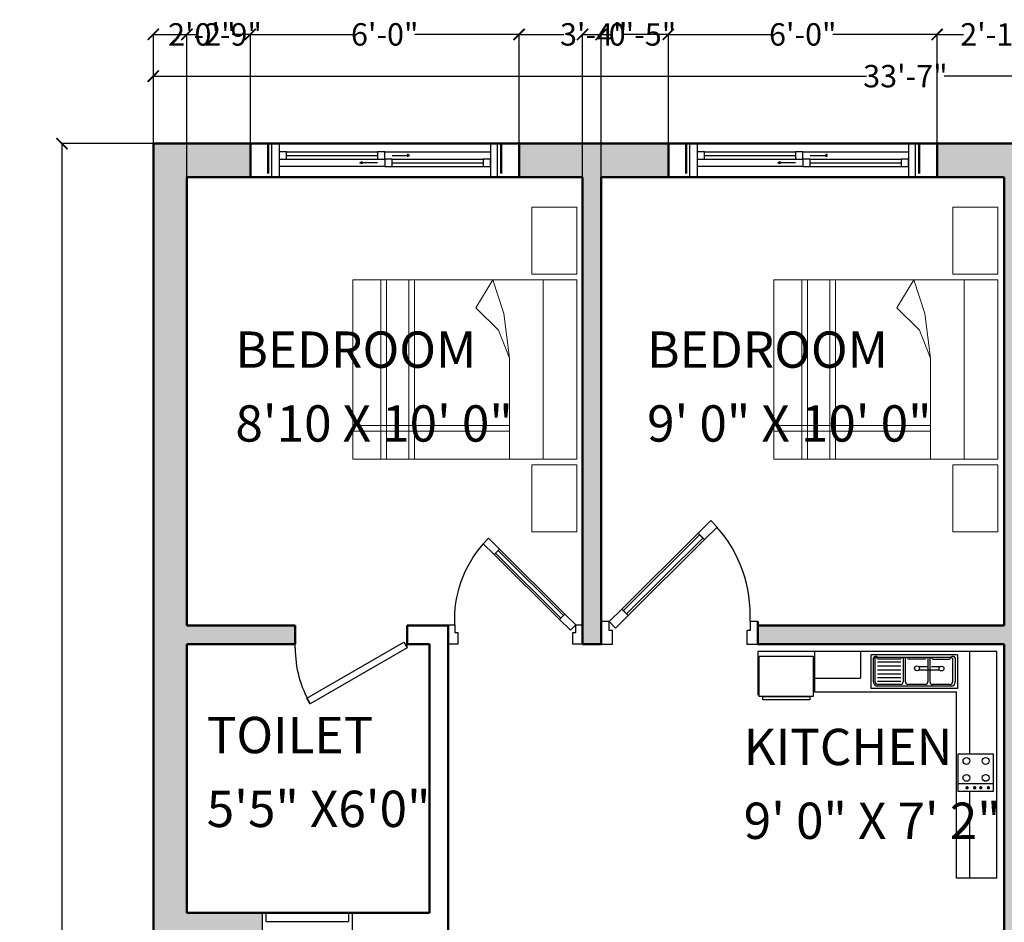
# Model space of a CAD drawing. Units: inches. Extents: x 2278 to 7495, y -71 to 1198.
# Tile 3 of 44: x 2278 to 2542, y 955 to 1197. Entities that reach past the tile are written whole.
import ezdxf

# ---------------------------------------------------------------- set-up
doc = ezdxf.new("R2010")
doc.units = ezdxf.units.IN
doc.header["$MEASUREMENT"] = 0
for name, color, linetype, lineweight in [('A-ANNO-DIMS', 2, 'Continuous', 18), ('A-AREA-IDEN', 3, 'Continuous', 18), ('A-Door', 3, 'Continuous', 25), ('A-FLOR-FIXT', 9, 'Continuous', 18), ('A-FURN', 8, 'Continuous', 18), ('A-Glaz', 4, 'Continuous', 25), ('A-Wall', 7, 'Continuous', 50), ('A-WALL-PATT', 8, 'Continuous', 18)]:
    doc.layers.add(name, color=color, linetype=linetype, lineweight=lineweight)
doc.layers.add('TEFRIŞ', color=11, linetype='Continuous')
doc.styles.get("Standard").update_dxf_attribs({"font": 'arial.ttf'})
doc.dimstyles.get("Standard").update_dxf_attribs({"dimtxt": 6, "dimasz": 3, "dimexe": 0.18, "dimexo": 0.0625, "dimgap": 0.09, "dimtad": 0, "dimtih": 1, "dimtoh": 1, "dimdec": 0, "dimzin": 0, "dimdsep": 46, "dimlunit": 3, "dimtxsty": 'Standard', "dimblk": 'ARCHTICK', "dimcen": 0.09, "dimadec": 0, "dimazin": 0, "dimtfac": 1, "dimtdec": 0, "dimtofl": 0, "dimtmove": 0, "dimatfit": 3, "dimfxl": 1, "dimtolj": 1, "dimtzin": 0, "dimarcsym": 0})

# ---------------------------------------------------------------- blocks, each defined once
blk = doc.blocks.new('A$C1DF4181C')
blk.add_lwpolyline([(120, 128), (460.7, 466.1), (432.5, 494.5), (91.8, 156.4)], close=True)
blk.add_arc((72.4, 128.7), 593.3, 357.2313, 41.4937)
at = {"layer": 'A-Door'}
for points in [[(517.5, 522.4), (460.7, 466.1), (432.5, 494.5), (489.3, 550.8)], [(63.2, 71.6), (120, 128), (91.8, 156.4), (35, 100)], [(35, 100), (0, 100), (0, 0), (50, 0), (50, 50), (50, 60), (35, 60)], [(665, 100), (665, 60), (650, 60), (650, 50), (650, 0), (700, 0), (700, 100)]]:
    blk.add_lwpolyline(points, close=True, dxfattribs=at)
at = {"layer": 'A-Glaz'}
blk.add_lwpolyline([(112.9, 135.1), (453.6, 473.2), (439.5, 487.4), (98.8, 149.3)], close=True, dxfattribs=at)
at = {"layer": 'A-Wall'}
for p, q in [((0, 0), (0, 100)), ((0, 100), (0, 0)), ((700, 0), (700, 100)), ((700, 0), (700, 100))]:
    blk.add_line(p, q, dxfattribs=at)
blk = doc.blocks.new('*U4')
for p, q in [((0, 0), (0, -6)), ((30, 0), (30, -6))]:
    blk.add_line(p, q)
blk.add_lwpolyline([(0, 0), (25.98, 15), (26.86, 13.48), (0.87, -1.52)], close=True)
blk.add_arc((0, 0), 30, 0, 30)
blk = doc.blocks.new('BED-160')
at = {"color": 0}
for p, q in [((-0.45, 2.35), (-0.45, 2.95)), ((-0.45, 2.95), (-0.05, 2.95)), ((-0.05, 2.95), (-0.05, 2.35)), ((-2.05, 2.3), (-0.05, 2.3)), ((-2.05, 0.7), (-2.05, 2.3)), ((-1.8, 0.7), (-1.8, 2.3)), ((-1.75, 0.7), (-1.75, 2.3)), ((-1.55, 0.7), (-1.55, 2.3)), ((-1.5, 0.7), (-1.5, 2.3)), ((-0.8, 2.3), (-0.95, 2.05)), ((-0.8, 2.3), (-0.7, 2)), ((-0.05, 2.35), (-0.45, 2.35)), ((-0.35, 0.7), (-0.35, 2.3)), ((-0.05, 2.3), (-0.05, 0.7)), ((-0.95, 2.05), (-0.75, 1.85)), ((-0.7, 2), (-0.65, 1.6)), ((-0.75, 1.85), (-0.65, 1.6)), ((-0.65, 1.6), (-0.65, 0.7)), ((-0.65, 1), (-2.05, 1)), ((-0.65, 0.95), (-2.05, 0.95)), ((-0.05, 0.7), (-2.05, 0.7)), ((-0.45, 0.65), (-0.05, 0.65)), ((-0.45, 0.05), (-0.45, 0.65)), ((-0.05, 0.65), (-0.05, 0.05)), ((-0.05, 0.05), (-0.45, 0.05))]:
    blk.add_line(p, q, dxfattribs=at)
blk = doc.blocks.new('A$C008029BD')
at = {"layer": 'TEFRIŞ', "ltscale": 0.05}
for p, q in [((0, 0), (0, -3.55)), ((3.37, 0), (0, 0)), ((3.37, 0), (3.37, -0.6)), ((1.522, -0.4), (0, -0.4)), ((3.37, -0.4), (2.083, -0.4)), ((0.05, -0.581), (0.05, -1.869)), ((0.05, -0.581), (0.55, -0.581)), ((0.55, -0.581), (0.55, -1.869)), ((0.086, -1.773), (0.086, -0.677)), ((0.096, -0.617), (0.454, -0.617)), ((0.099, -0.659), (0.457, -0.659)), ((0.113, -0.954), (0.113, -0.695)), ((0.493, -0.695), (0.493, -0.954)), ((0.514, -0.677), (0.514, -1.773)), ((0.6, -2.71), (0.6, -0.6)), ((3.37, -0.6), (0.6, -0.6)), ((0.23, -0.846), (0.229, -0.967)), ((0.28, -0.846), (0.277, -1.158)), ((0.096, -1.024), (0.454, -1.024)), ((0.457, -0.99), (0.099, -0.99)), ((0.228, -1.02), (0.227, -1.159)), ((0.11, -1.319), (0.11, -1.06)), ((0.49, -1.06), (0.49, -1.319)), ((0.454, -1.355), (0.096, -1.355)), ((0.096, -1.391), (0.454, -1.391)), ((0.11, -1.773), (0.11, -1.427)), ((0.154, -1.773), (0.154, -1.427)), ((0.214, -1.773), (0.214, -1.427)), ((0.274, -1.773), (0.274, -1.427)), ((0.334, -1.773), (0.334, -1.427)), ((0.39, -1.773), (0.39, -1.427)), ((0.444, -1.773), (0.444, -1.427)), ((0.49, -1.427), (0.49, -1.773)), ((0.55, -1.869), (0.05, -1.869)), ((0.454, -1.809), (0.096, -1.809)), ((0.454, -1.833), (0.096, -1.833)), ((0, -2.025), (0.4, -2.025)), ((0.4, -2.71), (0.4, -2.025)), ((0, -2.71), (0.6, -2.71)), ((0, -3.55), (0.65, -3.55))]:
    blk.add_line(p, q, dxfattribs=at)
at = {"layer": 'TEFRIŞ'}
blk.add_line((1.969, -0.05), (1.969, -0.572), dxfattribs=at)
at = {"layer": 'TEFRIŞ', "ltscale": 0.05}
for points in [[(1.522, -0.05), (2.083, -0.05), (2.083, -0.572), (1.522, -0.572)], [(0.67, -2.73), (0.67, -3.53), (0.07, -3.53), (0.07, -2.73)], [(0.72, -2.78), (0.72, -3.48), (0.67, -3.48), (0.67, -2.78)]]:
    blk.add_lwpolyline(points, close=True, dxfattribs=at)
at = {"layer": 'TEFRIŞ', "const_width": 0.025}
for points in [[(2.014, -0.123, 1), (2.039, -0.123, 1)], [(2.014, -0.236, 1), (2.039, -0.236, 1)], [(2.014, -0.327, 1), (2.039, -0.327, 1)], [(2.014, -0.44, 1), (2.039, -0.44, 1)]]:
    blk.add_lwpolyline(points, format="xyb", close=True, dxfattribs=at)
at = {"layer": 'TEFRIŞ', "ltscale": 0.05}
for centre, radius in [((1.628, -0.164), 0.0505), ((1.628, -0.45), 0.0505), ((0.255, -0.82), 0.036), ((0.252, -1.184), 0.036)]:
    blk.add_circle(centre, radius, dxfattribs=at)
at = {"layer": 'TEFRIŞ'}
for centre in [(1.88, -0.164), (1.88, -0.45)]:
    blk.add_circle(centre, 0.0505, dxfattribs=at)
at = {"layer": 'TEFRIŞ', "ltscale": 0.05}
for centre, radius, start, end in [((0.108, -0.649), 0.0351, 110.4976, 230.5777), ((0.118, -0.673), 0.023, 143.9853, 258.5157), ((0.454, -0.677), 0.06, 0, 90), ((0.457, -0.695), 0.036, 0, 90), ((0.115, -1.038), 0.023, 143.9853, 258.5157), ((0.118, -0.976), 0.023, 101.4843, 216.0147), ((0.454, -1.06), 0.036, 0, 90), ((0.457, -0.954), 0.036, 270, 0), ((0.115, -1.341), 0.023, 101.4843, 216.0147), ((0.115, -1.405), 0.023, 143.9853, 258.5157), ((0.454, -1.319), 0.036, 270, 0), ((0.454, -1.427), 0.036, 0, 90), ((0.108, -1.801), 0.0351, 129.4223, 249.5024), ((0.115, -1.796), 0.023, 101.4843, 216.0147), ((0.454, -1.773), 0.06, 270, 0), ((0.454, -1.773), 0.036, 270, 0)]:
    blk.add_arc(centre, radius, start, end, dxfattribs=at)
blk = doc.blocks.new('_ArchTick')
at = {"color": 0, "linetype": 'ByBlock', "const_width": 0.15}
blk.add_lwpolyline([(-0.5, -0.5), (0.5, 0.5)], dxfattribs=at)
blk = doc.blocks.new('*D17')
at = {"layer": 'A-ANNO-DIMS', "color": 0, "lineweight": -2, "transparency": 16777216}
for p, q in [((2313.81, 1163.47), (2289.2, 1163.47)), ((2289.38, 1163.47), (2289.38, 940.12)), ((2289.38, 710.47), (2289.38, 933.81)), ((2313.81, 710.47), (2289.2, 710.47))]:
    blk.add_line(p, q, dxfattribs=at)
at = {"layer": 'Defpoints', "color": 0, "transparency": 16777216}
for p in [(2313.87, 1163.47), (2289.38, 710.47), (2313.87, 710.47)]:
    blk.add_point(p, dxfattribs=at)
at = {"layer": 'A-ANNO-DIMS', "color": 0, "lineweight": -2, "transparency": 16777216, "xscale": 3, "yscale": 3, "zscale": 3}
for p, rotation in [((2289.38, 1163.47), 90), ((2289.38, 710.47), 270)]:
    blk.add_blockref('_ArchTick', p, dxfattribs=dict(at, rotation=rotation))
at = {"layer": 'A-ANNO-DIMS', "color": 0, "transparency": 16777216, "insert": (2289.38, 936.97), "char_height": 6, "attachment_point": 5}
blk.add_mtext('\\A1;37\'-9"', dxfattribs=at)
blk = doc.blocks.new('*D18')
at = {"layer": 'A-ANNO-DIMS', "color": 0, "lineweight": -2, "transparency": 16777216}
for p, q in [((2313.87, 1163.53), (2313.87, 1181.72)), ((2313.87, 1181.54), (2504.98, 1181.54)), ((2716.87, 1181.54), (2525.76, 1181.54)), ((2716.87, 1163.53), (2716.87, 1181.72))]:
    blk.add_line(p, q, dxfattribs=at)
at = {"layer": 'Defpoints', "color": 0, "transparency": 16777216}
for p in [(2716.87, 1181.54), (2313.87, 1163.47), (2716.87, 1163.47)]:
    blk.add_point(p, dxfattribs=at)
at = {"layer": 'A-ANNO-DIMS', "color": 0, "lineweight": -2, "transparency": 16777216, "xscale": 3, "yscale": 3, "zscale": 3, "rotation": 180}
blk.add_blockref('_ArchTick', (2313.87, 1181.54), dxfattribs=at)
at = {"layer": 'A-ANNO-DIMS', "color": 0, "lineweight": -2, "transparency": 16777216, "xscale": 3, "yscale": 3, "zscale": 3}
blk.add_blockref('_ArchTick', (2716.87, 1181.54), dxfattribs=at)
at = {"layer": 'A-ANNO-DIMS', "color": 0, "transparency": 16777216, "insert": (2515.37, 1181.54), "char_height": 6, "attachment_point": 5}
blk.add_mtext('\\A1;33\'-7"', dxfattribs=at)
blk = doc.blocks.new('*D61')
at = {"layer": 'A-ANNO-DIMS', "color": 0, "lineweight": -2, "transparency": 16777216}
for p, q in [((2313.87, 1163.53), (2313.87, 1192.9)), ((2313.87, 1192.72), (2318.75, 1192.72)), ((2339.87, 1192.72), (2334.99, 1192.72)), ((2339.87, 1163.53), (2339.87, 1192.9))]:
    blk.add_line(p, q, dxfattribs=at)
at = {"layer": 'Defpoints', "color": 0, "transparency": 16777216}
for p in [(2339.87, 1192.72), (2313.87, 1163.47), (2339.87, 1163.47)]:
    blk.add_point(p, dxfattribs=at)
at = {"layer": 'A-ANNO-DIMS', "color": 0, "lineweight": -2, "transparency": 16777216, "xscale": 3, "yscale": 3, "zscale": 3, "rotation": 180}
blk.add_blockref('_ArchTick', (2313.87, 1192.72), dxfattribs=at)
at = {"layer": 'A-ANNO-DIMS', "color": 0, "lineweight": -2, "transparency": 16777216, "xscale": 3, "yscale": 3, "zscale": 3}
blk.add_blockref('_ArchTick', (2339.87, 1192.72), dxfattribs=at)
at = {"layer": 'A-ANNO-DIMS', "color": 0, "transparency": 16777216, "insert": (2326.87, 1192.72), "char_height": 6, "attachment_point": 5}
blk.add_mtext('\\A1;2\'-2"', dxfattribs=at)
blk = doc.blocks.new('*D62')
at = {"layer": 'A-ANNO-DIMS', "color": 0, "lineweight": -2, "transparency": 16777216}
for p, q in [((2339.87, 1163.53), (2339.87, 1192.9)), ((2339.87, 1192.72), (2367.79, 1192.72)), ((2411.87, 1192.72), (2383.95, 1192.72)), ((2411.87, 1163.53), (2411.87, 1192.9))]:
    blk.add_line(p, q, dxfattribs=at)
at = {"layer": 'Defpoints', "color": 0, "transparency": 16777216}
for p in [(2411.87, 1192.72), (2339.87, 1163.47), (2411.87, 1163.47)]:
    blk.add_point(p, dxfattribs=at)
at = {"layer": 'A-ANNO-DIMS', "color": 0, "lineweight": -2, "transparency": 16777216, "xscale": 3, "yscale": 3, "zscale": 3, "rotation": 180}
blk.add_blockref('_ArchTick', (2339.87, 1192.72), dxfattribs=at)
at = {"layer": 'A-ANNO-DIMS', "color": 0, "lineweight": -2, "transparency": 16777216, "xscale": 3, "yscale": 3, "zscale": 3}
blk.add_blockref('_ArchTick', (2411.87, 1192.72), dxfattribs=at)
at = {"layer": 'A-ANNO-DIMS', "color": 0, "transparency": 16777216, "insert": (2375.87, 1192.72), "char_height": 6, "attachment_point": 5}
blk.add_mtext('\\A1;6\'-0"', dxfattribs=at)
blk = doc.blocks.new('*D63')
at = {"layer": 'A-ANNO-DIMS', "color": 0, "lineweight": -2, "transparency": 16777216}
for p, q in [((2411.87, 1163.53), (2411.87, 1192.9)), ((2411.87, 1192.72), (2423.81, 1192.72)), ((2451.87, 1192.72), (2439.93, 1192.72)), ((2451.87, 1163.53), (2451.87, 1192.9))]:
    blk.add_line(p, q, dxfattribs=at)
at = {"layer": 'Defpoints', "color": 0, "transparency": 16777216}
for p in [(2451.87, 1192.72), (2411.87, 1163.47), (2451.87, 1163.47)]:
    blk.add_point(p, dxfattribs=at)
at = {"layer": 'A-ANNO-DIMS', "color": 0, "lineweight": -2, "transparency": 16777216, "xscale": 3, "yscale": 3, "zscale": 3, "rotation": 180}
blk.add_blockref('_ArchTick', (2411.87, 1192.72), dxfattribs=at)
at = {"layer": 'A-ANNO-DIMS', "color": 0, "lineweight": -2, "transparency": 16777216, "xscale": 3, "yscale": 3, "zscale": 3}
blk.add_blockref('_ArchTick', (2451.87, 1192.72), dxfattribs=at)
at = {"layer": 'A-ANNO-DIMS', "color": 0, "transparency": 16777216, "insert": (2431.87, 1192.72), "char_height": 6, "attachment_point": 5}
blk.add_mtext('\\A1;3\'-4"', dxfattribs=at)
blk = doc.blocks.new('*D64')
at = {"layer": 'A-ANNO-DIMS', "color": 0, "lineweight": -2, "transparency": 16777216}
for p, q in [((2451.87, 1163.53), (2451.87, 1192.9)), ((2451.87, 1192.72), (2479.79, 1192.72)), ((2523.87, 1192.72), (2495.95, 1192.72)), ((2523.87, 1163.53), (2523.87, 1192.9))]:
    blk.add_line(p, q, dxfattribs=at)
at = {"layer": 'Defpoints', "color": 0, "transparency": 16777216}
for p in [(2523.87, 1192.72), (2451.87, 1163.47), (2523.87, 1163.47)]:
    blk.add_point(p, dxfattribs=at)
at = {"layer": 'A-ANNO-DIMS', "color": 0, "lineweight": -2, "transparency": 16777216, "xscale": 3, "yscale": 3, "zscale": 3, "rotation": 180}
blk.add_blockref('_ArchTick', (2451.87, 1192.72), dxfattribs=at)
at = {"layer": 'A-ANNO-DIMS', "color": 0, "lineweight": -2, "transparency": 16777216, "xscale": 3, "yscale": 3, "zscale": 3}
blk.add_blockref('_ArchTick', (2523.87, 1192.72), dxfattribs=at)
at = {"layer": 'A-ANNO-DIMS', "color": 0, "transparency": 16777216, "insert": (2487.87, 1192.72), "char_height": 6, "attachment_point": 5}
blk.add_mtext('\\A1;6\'-0"', dxfattribs=at)
blk = doc.blocks.new('*D65')
at = {"layer": 'A-ANNO-DIMS', "color": 0, "lineweight": -2, "transparency": 16777216}
for p, q in [((2523.87, 1163.53), (2523.87, 1192.9)), ((2523.87, 1192.72), (2530.92, 1192.72)), ((2558.87, 1192.72), (2551.82, 1192.72)), ((2558.87, 1163.53), (2558.87, 1192.9))]:
    blk.add_line(p, q, dxfattribs=at)
at = {"layer": 'Defpoints', "color": 0, "transparency": 16777216}
for p in [(2558.87, 1192.72), (2523.87, 1163.47), (2558.87, 1163.47)]:
    blk.add_point(p, dxfattribs=at)
at = {"layer": 'A-ANNO-DIMS', "color": 0, "lineweight": -2, "transparency": 16777216, "xscale": 3, "yscale": 3, "zscale": 3, "rotation": 180}
blk.add_blockref('_ArchTick', (2523.87, 1192.72), dxfattribs=at)
at = {"layer": 'A-ANNO-DIMS', "color": 0, "lineweight": -2, "transparency": 16777216, "xscale": 3, "yscale": 3, "zscale": 3}
blk.add_blockref('_ArchTick', (2558.87, 1192.72), dxfattribs=at)
at = {"layer": 'A-ANNO-DIMS', "color": 0, "transparency": 16777216, "insert": (2541.37, 1192.72), "char_height": 6, "attachment_point": 5}
blk.add_mtext('\\A1;2\'-11"', dxfattribs=at)
blk = doc.blocks.new('*D75')
at = {"layer": 'A-ANNO-DIMS', "color": 0, "lineweight": -2, "transparency": 16777216}
for p, q in [((2313.87, 1163.53), (2313.87, 1192.9)), ((2313.87, 1192.72), (2322.87, 1192.72)), ((2322.87, 1154.53), (2322.87, 1192.9)), ((2322.87, 1192.72), (2325.87, 1192.72))]:
    blk.add_line(p, q, dxfattribs=at)
at = {"layer": 'Defpoints', "color": 0, "transparency": 16777216}
for p in [(2322.87, 1192.72), (2313.87, 1163.47), (2322.87, 1154.47)]:
    blk.add_point(p, dxfattribs=at)
at = {"layer": 'A-ANNO-DIMS', "color": 0, "lineweight": -2, "transparency": 16777216, "xscale": 3, "yscale": 3, "zscale": 3, "rotation": 180}
blk.add_blockref('_ArchTick', (2313.87, 1192.72), dxfattribs=at)
at = {"layer": 'A-ANNO-DIMS', "color": 0, "lineweight": -2, "transparency": 16777216, "xscale": 3, "yscale": 3, "zscale": 3}
blk.add_blockref('_ArchTick', (2322.87, 1192.72), dxfattribs=at)
at = {"layer": 'A-ANNO-DIMS', "color": 0, "transparency": 16777216, "insert": (2333.93, 1192.72), "char_height": 6, "attachment_point": 5}
blk.add_mtext('\\A1;0\'-9"', dxfattribs=at)
blk = doc.blocks.new('*D76')
at = {"layer": 'A-ANNO-DIMS', "color": 0, "lineweight": -2, "transparency": 16777216}
for p, q in [((2428.87, 1029.53), (2428.87, 1192.9)), ((2428.87, 1192.72), (2433.87, 1192.72)), ((2433.87, 1029.53), (2433.87, 1192.9)), ((2433.87, 1192.72), (2436.87, 1192.72))]:
    blk.add_line(p, q, dxfattribs=at)
at = {"layer": 'Defpoints', "color": 0, "transparency": 16777216}
for p in [(2433.87, 1192.72), (2428.87, 1029.47), (2433.87, 1029.47)]:
    blk.add_point(p, dxfattribs=at)
at = {"layer": 'A-ANNO-DIMS', "color": 0, "lineweight": -2, "transparency": 16777216, "xscale": 3, "yscale": 3, "zscale": 3, "rotation": 180}
blk.add_blockref('_ArchTick', (2428.87, 1192.72), dxfattribs=at)
at = {"layer": 'A-ANNO-DIMS', "color": 0, "lineweight": -2, "transparency": 16777216, "xscale": 3, "yscale": 3, "zscale": 3}
blk.add_blockref('_ArchTick', (2433.87, 1192.72), dxfattribs=at)
at = {"layer": 'A-ANNO-DIMS', "color": 0, "transparency": 16777216, "insert": (2444.93, 1192.72), "char_height": 6, "attachment_point": 5}
blk.add_mtext('\\A1;0\'-5"', dxfattribs=at)

msp = doc.modelspace()

# ---------------------------------------------------------------- hatches: boundary and pattern name
at = {"layer": 'A-WALL-PATT'}
h = msp.add_hatch(dxfattribs=at)
h.set_pattern_fill('ANSI36', color=256, scale=30)
h.paths.add_polyline_path([(2343.12, 957.47), (2322.87, 957.47), (2322.87, 1029.47), (2351.87, 1029.47), (2351.87, 1034.47), (2322.87, 1034.47), (2322.87, 1154.47), (2339.87, 1154.47), (2339.87, 1163.47), (2313.87, 1163.47), (2313.87, 710.47), (2445.87, 710.47), (2445.87, 719.47), (2322.87, 719.47), (2322.87, 807.47), (2404.87, 807.47), (2404.87, 812.47), (2392.87, 812.47), (2392.87, 881.47), (2387.87, 881.47), (2387.87, 812.47), (2322.87, 812.47), (2322.87, 911.47), (2345.87, 911.47), (2345.87, 916.47), (2322.87, 916.47), (2322.87, 952.47), (2343.12, 952.47)])
h.paths.add_polyline_path([(2451.87, 1163.47), (2411.87, 1163.47), (2411.87, 1154.47), (2428.87, 1154.47), (2428.87, 1034.47), (2428.87, 1029.47), (2433.87, 1029.47), (2433.87, 1154.47), (2451.87, 1154.47)])
h.paths.add_polyline_path([(2558.87, 1163.47), (2523.87, 1163.47), (2523.87, 1154.47), (2541.87, 1154.47), (2541.87, 1034.47), (2475.87, 1034.47), (2475.87, 1029.47), (2541.87, 1029.47), (2541.87, 943.47), (2541.87, 940.13), (2541.87, 876.47), (2493.87, 876.47), (2493.87, 943.47), (2488.87, 943.47), (2488.87, 871.47), (2488.87, 865.74), (2493.88, 865.74), (2493.88, 871.47), (2541.87, 871.47), (2541.87, 805.47), (2546.87, 805.47), (2546.87, 1077.47), (2558.87, 1077.47), (2558.87, 1082.47), (2546.87, 1082.47), (2546.87, 1154.47), (2558.87, 1154.47)])
h.paths.add_polyline_path([(2716.87, 937.97), (2707.87, 937.97), (2707.87, 911.47), (2594.87, 911.47), (2594.87, 906.47), (2707.87, 906.47), (2707.87, 869.47), (2716.87, 869.47)])
h.paths.add_polyline_path([(2716.87, 1163.47), (2689.87, 1163.47), (2689.87, 1154.47), (2707.87, 1154.47), (2707.87, 1041.47), (2594.87, 1041.47), (2594.87, 1036.47), (2707.87, 1036.47), (2707.87, 1009.97), (2716.87, 1009.97)])
h.paths.add_polyline_path([(2617.87, 1163.47), (2582.87, 1163.47), (2582.87, 1154.47), (2594.87, 1154.47), (2594.87, 1082.47), (2588.87, 1082.47), (2588.87, 1077.47), (2599.87, 1077.47), (2599.87, 1154.47), (2617.87, 1154.47)])
h.paths.add_polyline_path([(2716.87, 797.47), (2707.87, 797.47), (2707.87, 760.47), (2663.37, 760.47), (2663.37, 755.47), (2716.87, 755.47)])
h.paths.add_polyline_path([(2591.37, 760.47), (2546.87, 760.47), (2546.87, 763.47), (2541.87, 763.47), (2541.87, 755.47), (2591.37, 755.47)])

# ---------------------------------------------------------------- linework, layer by layer
at = {"layer": 'A-Glaz'}
for p, q in [((2347.57, 1163.47), (2404.17, 1163.47)), ((2459.57, 1163.47), (2516.17, 1163.47)), ((2349.52, 1161.3), (2373.92, 1161.3)), ((2375.87, 1161.3), (2404.17, 1161.3)), ((2461.52, 1161.3), (2485.92, 1161.3)), ((2487.87, 1161.3), (2516.17, 1161.3)), ((2349.52, 1160.32), (2373.92, 1160.32)), ((2349.52, 1159.35), (2373.92, 1159.35)), ((2373.92, 1158.37), (2369.73, 1158.37)), ((2377.82, 1160.32), (2382.01, 1160.32)), ((2377.82, 1159.35), (2402.22, 1159.35)), ((2377.82, 1158.37), (2402.22, 1158.37)), ((2461.52, 1160.32), (2485.92, 1160.32)), ((2461.52, 1159.35), (2485.92, 1159.35)), ((2485.92, 1158.37), (2481.73, 1158.37)), ((2489.82, 1160.32), (2494.01, 1160.32)), ((2489.82, 1159.35), (2514.22, 1159.35)), ((2489.82, 1158.37), (2514.22, 1158.37)), ((2375.87, 1157.39), (2347.57, 1157.39)), ((2377.82, 1157.39), (2402.22, 1157.39)), ((2487.87, 1157.39), (2459.57, 1157.39)), ((2489.82, 1157.39), (2514.22, 1157.39)), ((2347.57, 1154.47), (2404.17, 1154.47)), ((2459.57, 1154.47), (2516.17, 1154.47)), ((2343.12, 957.47), (2367.12, 957.47)), ((2343.12, 952.47), (2343.12, 957.47)), ((2344.12, 955.17), (2344.12, 957.47)), ((2344.12, 955.17), (2366.12, 955.17)), ((2366.12, 957.47), (2366.12, 955.17)), ((2367.12, 957.47), (2367.12, 952.47))]:
    msp.add_line(p, q, dxfattribs=at)
for points in [[(2347.57, 1154.47), (2345.62, 1154.47), (2345.62, 1163.47), (2347.57, 1163.47)], [(2404.17, 1154.47), (2406.12, 1154.47), (2406.12, 1163.47), (2404.17, 1163.47)], [(2459.57, 1154.47), (2457.62, 1154.47), (2457.62, 1163.47), (2459.57, 1163.47)], [(2516.17, 1154.47), (2518.12, 1154.47), (2518.12, 1163.47), (2516.17, 1163.47)], [(2347.57, 1159.35), (2349.52, 1159.35), (2349.52, 1161.3), (2347.57, 1161.3)], [(2373.92, 1159.35), (2375.87, 1159.35), (2375.87, 1161.3), (2373.92, 1161.3)], [(2459.57, 1159.35), (2461.52, 1159.35), (2461.52, 1161.3), (2459.57, 1161.3)], [(2485.92, 1159.35), (2487.87, 1159.35), (2487.87, 1161.3), (2485.92, 1161.3)], [(2369.22, 1158.37), (2369.73, 1158.66), (2369.73, 1158.08)], [(2375.87, 1157.39), (2377.82, 1157.39), (2377.82, 1159.35), (2375.87, 1159.35)], [(2382.52, 1160.32), (2382.01, 1160.61), (2382.01, 1160.03)], [(2402.22, 1157.39), (2404.17, 1157.39), (2404.17, 1159.35), (2402.22, 1159.35)], [(2481.22, 1158.37), (2481.73, 1158.66), (2481.73, 1158.08)], [(2487.87, 1157.39), (2489.82, 1157.39), (2489.82, 1159.35), (2487.87, 1159.35)], [(2494.52, 1160.32), (2494.01, 1160.61), (2494.01, 1160.03)], [(2514.22, 1157.39), (2516.17, 1157.39), (2516.17, 1159.35), (2514.22, 1159.35)]]:
    msp.add_lwpolyline(points, close=True, dxfattribs=at)
at = {"layer": 'A-Wall'}
for p, q in [((2313.87, 1163.47), (2313.87, 710.47)), ((2313.87, 1163.47), (2716.87, 1163.47)), ((2339.87, 1154.47), (2339.87, 1163.47)), ((2345.62, 1163.47), (2339.87, 1163.47)), ((2406.12, 1163.47), (2411.87, 1163.47)), ((2411.87, 1154.47), (2411.87, 1163.47)), ((2451.87, 1154.47), (2451.87, 1163.47)), ((2457.62, 1163.47), (2451.87, 1163.47)), ((2518.12, 1163.47), (2523.87, 1163.47)), ((2523.87, 1154.47), (2523.87, 1163.47)), ((2344.64, 1163.25), (2344.64, 1155.44)), ((2407.1, 1163.25), (2407.1, 1155.44)), ((2456.64, 1163.25), (2456.64, 1155.44)), ((2519.1, 1163.25), (2519.1, 1155.44)), ((2322.87, 1154.47), (2322.87, 1034.47)), ((2322.87, 1154.47), (2428.87, 1154.47)), ((2345.62, 1154.47), (2339.87, 1154.47)), ((2406.12, 1154.47), (2411.87, 1154.47)), ((2428.87, 1154.47), (2428.87, 1034.47)), ((2433.87, 1154.47), (2433.87, 1029.47)), ((2433.87, 1154.47), (2541.87, 1154.47)), ((2457.62, 1154.47), (2451.87, 1154.47)), ((2518.12, 1154.47), (2523.87, 1154.47)), ((2541.87, 1154.47), (2541.87, 1034.47)), ((2322.87, 1034.47), (2351.87, 1034.47)), ((2351.87, 1029.47), (2351.87, 1034.47)), ((2381.87, 1029.47), (2381.87, 1034.47)), ((2381.87, 1034.47), (2392.87, 1034.47)), ((2392.87, 1034.47), (2392.87, 1029.47)), ((2428.87, 1034.47), (2428.87, 1029.47)), ((2475.87, 1034.47), (2541.87, 1034.47)), ((2475.87, 1029.47), (2475.87, 1034.47)), ((2322.87, 1029.47), (2351.87, 1029.47)), ((2322.87, 1029.47), (2322.87, 957.47)), ((2381.87, 1029.47), (2387.87, 1029.47)), ((2387.87, 1029.47), (2387.87, 957.47)), ((2392.87, 1029.47), (2392.87, 911.47)), ((2428.87, 1029.47), (2433.87, 1029.47)), ((2475.87, 1029.47), (2541.87, 1029.47)), ((2541.87, 1029.47), (2541.87, 943.47)), ((2322.87, 957.47), (2387.87, 957.47))]:
    msp.add_line(p, q, dxfattribs=at)

# ---------------------------------------------------------------- block references
at = {"layer": 'A-Door'}
for p, xscale, yscale, zscale in [((2433.87, 1029.47), 0.0599999999999766, 0.0599999999999766, 0.0599999999999766), ((2428.87, 1029.47), -0.051428571401403, 0.051428571401403, 0.051428571401403)]:
    msp.add_blockref('A$C1DF4181C', p, dxfattribs=dict(at, xscale=xscale, yscale=yscale, zscale=zscale))
at = {"layer": 'A-Door', "rotation": 180}
msp.add_blockref('*U4', (2381.87, 1028.47), dxfattribs=at)
at = {"layer": 'A-FLOR-FIXT', "xscale": 18.01737512370223, "yscale": 18.01737512370223, "zscale": 18.01737512370223, "rotation": 270}
msp.add_blockref('A$C008029BD', (2539.83, 1027.5), dxfattribs=at)
at = {"layer": 'A-FURN', "xscale": 29.9999999999997, "yscale": 29.9999999999997, "zscale": 29.9999999999997}
for p in [(2428.82, 1058), (2541.61, 1058)]:
    msp.add_blockref('BED-160', p, dxfattribs=at)

# ---------------------------------------------------------------- texts
at = {"layer": 'A-AREA-IDEN'}
for s, height, p in [('BEDROOM', 9.72, (2335.86, 1103.45)), ('BEDROOM', 9.72, (2446.16, 1103.45)), ('8\'10 X 10\' 0"', 9.7203, (2335.86, 1083.68)), ('9\' 0" X 10\' 0"', 9.7203, (2446.16, 1083.68)), ('TOILET', 9.72, (2328.18, 1000.25)), ('KITCHEN', 9.72, (2472.05, 997.06)), ('5\'5" X6\'0"', 9.72, (2328.18, 980.48)), ('9\' 0" X 7\' 2"', 9.7203, (2472.05, 977.29))]:
    msp.add_text(s, height=height, dxfattribs=at).set_placement(p)

# ---------------------------------------------------------------- dimensions: what is measured, and where the dimension line sits
at = {"layer": 'A-ANNO-DIMS'}
for base, p1, p2, override, picture, middle in [((2339.87, 1192.72), (2313.87, 1163.47), (2339.87, 1163.47), {"dimdec": 1, "dimlfac": 1, "dimrnd": 0, "dimzin": 1, "dimdsep": 46, "dimlunit": 4, "dimfrac": 2}, '*D61', (2326.87, 1192.72)), ((2322.87, 1192.72), (2313.87, 1163.47), (2322.87, 1154.47), {"dimdec": 1, "dimlfac": 1, "dimrnd": 0, "dimzin": 1, "dimdsep": 46, "dimlunit": 4, "dimfrac": 2}, '*D75', (2333.93, 1192.72)), ((2411.87, 1192.72), (2339.87, 1163.47), (2411.87, 1163.47), {"dimdec": 1, "dimlfac": 1, "dimrnd": 0, "dimzin": 1, "dimdsep": 46, "dimlunit": 4, "dimfrac": 2}, '*D62', (2375.87, 1192.72)), ((2451.87, 1192.72), (2411.87, 1163.47), (2451.87, 1163.47), {"dimdec": 1, "dimlfac": 1, "dimrnd": 0, "dimzin": 1, "dimdsep": 46, "dimlunit": 4, "dimfrac": 2}, '*D63', (2431.87, 1192.72)), ((2433.87, 1192.72), (2428.87, 1029.47), (2433.87, 1029.47), {"dimdec": 1, "dimlfac": 1, "dimrnd": 0, "dimzin": 1, "dimdsep": 46, "dimlunit": 4, "dimfrac": 2}, '*D76', (2444.93, 1192.72)), ((2523.87, 1192.72), (2451.87, 1163.47), (2523.87, 1163.47), {"dimdec": 1, "dimlfac": 1, "dimrnd": 0, "dimzin": 1, "dimdsep": 46, "dimlunit": 4, "dimfrac": 2}, '*D64', (2487.87, 1192.72)), ((2558.87, 1192.72), (2523.87, 1163.47), (2558.87, 1163.47), {"dimdec": 1, "dimlfac": 1, "dimrnd": 0, "dimzin": 1, "dimdsep": 46, "dimlunit": 4, "dimfrac": 2}, '*D65', (2541.37, 1192.72)), ((2716.87, 1181.54), (2313.87, 1163.47), (2716.87, 1163.47), {"dimclrd": 0, "dimclre": 0, "dimclrt": 0}, '*D18', (2515.37, 1181.54))]:
    dim = msp.add_linear_dim(base=base, p1=p1, p2=p2, dimstyle='Standard', override=override, dxfattribs=at)
    dim.commit()
    dim.dimension.update_dxf_attribs({"geometry": picture, "text_midpoint": middle})
dim = msp.add_linear_dim(base=(2289.38, 710.47), p1=(2313.87, 1163.47), p2=(2313.87, 710.47), angle=90, dimstyle='Standard', override={"dimclrd": 0, "dimclre": 0, "dimclrt": 0}, dxfattribs=at)
dim.commit()
dim.dimension.update_dxf_attribs({"geometry": '*D17', "text_midpoint": (2289.38, 936.97)})

doc.saveas('drawing.dxf')
